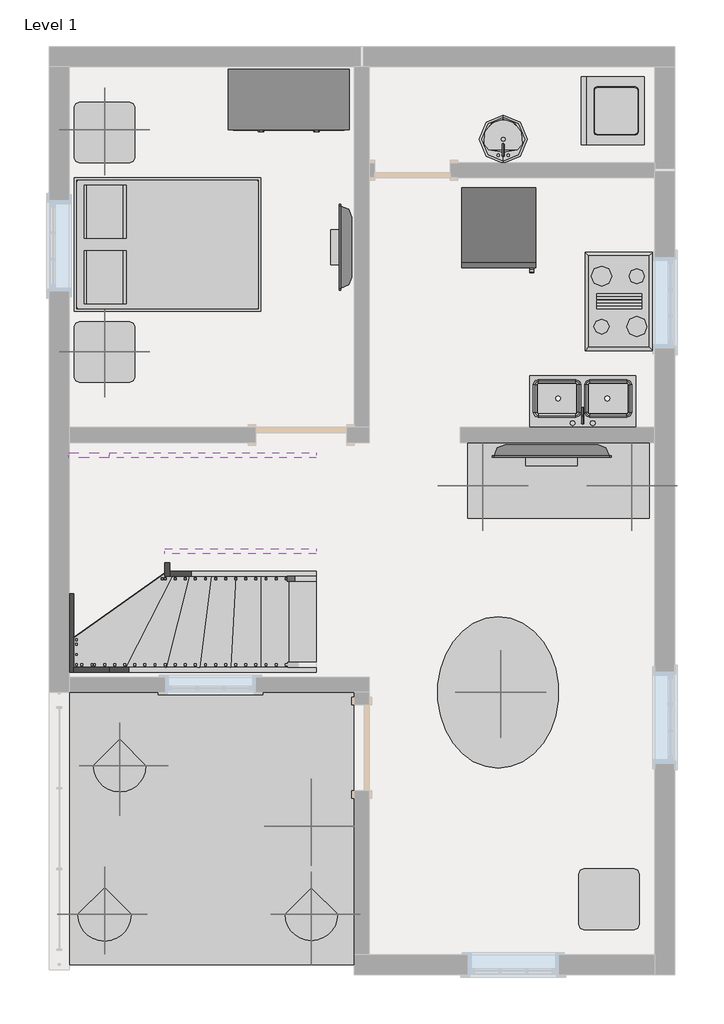
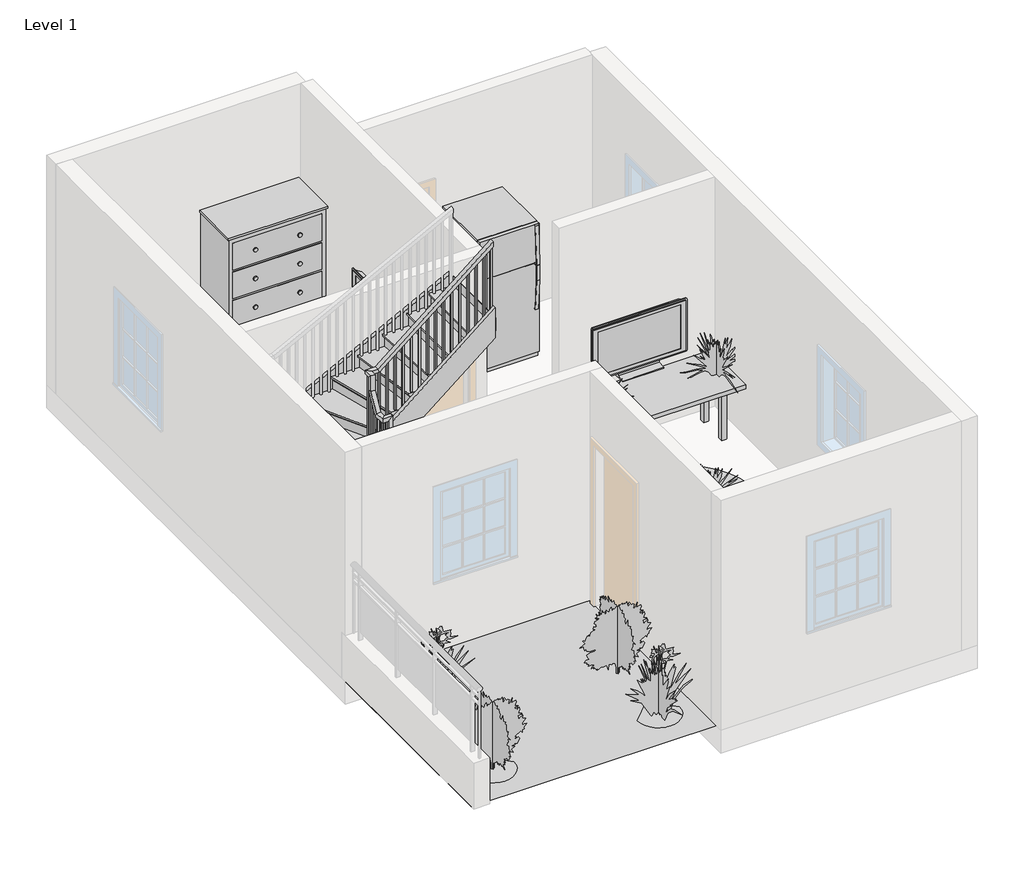
# One storey, part 3 of 3: 9 furniture elements, 9 geographic elements, 8 members, 4 proxies, 3 flow terminals, 1 railing, 1 stair flight.
"""IFC4 building model written with IfcOpenShell, lengths in millimetres."""

from ifc_helpers import new_model, si_unit, frame, origin, place, context, project, spatial, polyline, outline, extrude, faceted_brep, triangles, transform, mapped, element, save
from components import proxy_bb1e6e30, proxy_a13a33b2, proxy_718fa39f, flow_terminal_2b63360b, flow_terminal_a53be723, flow_terminal_d49f872f, furniture_c8abb964, furniture_9fa109b2, furniture_56245f3a, furniture_d9bcc661, furniture_743965d2, furniture_31d08a24, furniture_a5b052b6, rpc_plant_tropical_55f6ff97, rpc_plant_tropical_agave_1_5_93a2a214, rpc_plant_tropical_jungle_flame_3_9c4808c2, stair_flight_e7c1aa98

model = new_model("IFC4")

# Units and contexts
model_context = context("Model", 3, world=origin())
ifc_project = project(units=[si_unit("LENGTHUNIT", "METRE", prefix="MILLI")], contexts=[model_context])

# Site, building, storey
site = spatial("IfcSite", under=ifc_project)
building = spatial("IfcBuilding", under=site)
storey = spatial("IfcBuildingStorey", under=building, Name="Level 1", Elevation=0.0)

# Proxies
placement = place(None, origin())
element("IfcBuildingElementProxy", 1, Name="Building Element Proxy", at=placement, inside=storey, context=model_context, shape_type="Tessellation", body=[
    triangles([(-16784.817334, 6612.6463715, 0.0), (-13559.0165588, 6487.3377411, 0.0), (-13635.2165588, 3869.4466621, 0.0), (-16784.817334, 3869.4466621, 0.0), (-13711.4165588, 6612.6463715, 0.0)], [[1, 4, 5], [5, 3, 2], [3, 5, 4]], closed=False),
])
proxy_shape = proxy_bb1e6e30(model_context)
element("IfcBuildingElementProxy", 2, Name="Cook Top-4 Unit : 36\" x 20\"", ObjectType="Cook Top-4 Unit : 36\" x 20\"", at=placement, inside=storey, context=model_context, shape_type="MappedRepresentation", body=[
    mapped(proxy_shape, transform((-11044.4170266, 10549.6465295, 0.0), x_axis=(0.0, -1.0000000000000004, 0.0), y_axis=(1.0000000000000004, 0.0, 0.0), z_axis=(0.0, 0.0, 1.0))),
])
proxy_2_shape = proxy_a13a33b2(model_context)
element("IfcBuildingElementProxy", 3, Name="Refrigerator : 30\" x 32\" RH", ObjectType="Refrigerator : 30\" x 32\" RH", at=placement, inside=storey, context=model_context, shape_type="MappedRepresentation", body=[
    mapped(proxy_2_shape, transform((-12255.6795266, 11304.097558, 0.0), x_axis=(1.0, 0.0, 0.0), y_axis=(0.0, 1.0, 0.0), z_axis=(0.0, 0.0, 1.0))),
])
proxy_3_shape = proxy_718fa39f(model_context)
element("IfcBuildingElementProxy", 4, Name="Washer : 27\" x 25\" x 35\"", ObjectType="Washer : 27\" x 25\" x 35\"", at=placement, inside=storey, context=model_context, shape_type="MappedRepresentation", body=[
    mapped(proxy_3_shape, transform((-10828.7674618, 12046.929061, 0.0), x_axis=(0.0, 1.0000000000000002, 0.0), y_axis=(-1.0000000000000002, 0.0, 0.0), z_axis=(0.0, 0.0, 1.0))),
])

# Flow terminals
flow_terminal_shape = flow_terminal_2b63360b(model_context)
element("IfcFlowTerminal", 5, ObjectType="Floor Drain - Rectangular : 5\"x5\" Strainer - 2\" Drain", at=placement, inside=storey, context=model_context, shape_type="MappedRepresentation", body=[
    mapped(flow_terminal_shape, transform((-11806.4170266, 12734.0465295, 0.0), x_axis=(1.0, 0.0, 0.0), y_axis=(0.0, 1.0, 0.0), z_axis=(0.0, 0.0, 1.0))),
])
flow_terminal_2_shape = flow_terminal_a53be723(model_context)
element("IfcFlowTerminal", 6, ObjectType="Sink Kitchen-Double : 42\" x 21\"", at=placement, inside=storey, context=model_context, shape_type="MappedRepresentation", body=[
    mapped(flow_terminal_2_shape, transform((-11397.027786, 9535.9919306, 0.0), x_axis=(-1.0, 0.0, 0.0), y_axis=(0.0, -1.0, 0.0), z_axis=(0.0, 0.0, 1.0))),
])
flow_terminal_3_shape = flow_terminal_d49f872f(model_context)
element("IfcFlowTerminal", 7, ObjectType="Sink Vanity-Round : 19\" x 19\"", at=placement, inside=storey, context=model_context, shape_type="MappedRepresentation", body=[
    mapped(flow_terminal_3_shape, transform((-12116.165286, 12267.8503956, 0.0), x_axis=(-1.0000000000000004, 0.0, 0.0), y_axis=(0.0, -1.0000000000000004, 0.0), z_axis=(0.0, 0.0, 1.0))),
])

# Furniture
furniture_shape = furniture_c8abb964(model_context)
element("IfcFurniture", 8, ObjectType="Bed-Box : Double 53\" x 74\"", at=placement, inside=storey, context=model_context, shape_type="MappedRepresentation", body=[
    mapped(furniture_shape, transform((-15825.4465348, 10781.9940704, 0.0), x_axis=(0.0, 1.0, 0.0), y_axis=(-1.0, 0.0, 0.0), z_axis=(0.0, 0.0, 1.0))),
])
furniture_2_shape = furniture_9fa109b2(model_context)
element("IfcFurniture", 9, ObjectType="Dresser : 48\" x 72\" x 24\"", at=placement, inside=storey, context=model_context, shape_type="MappedRepresentation", body=[
    mapped(furniture_2_shape, transform((-14102.6237667, 12944.8094836, 0.0), x_axis=(1.0, 0.0, 0.0), y_axis=(0.0, 1.0, 0.0), z_axis=(0.0, 0.0, 1.0))),
])
furniture_3_shape = furniture_56245f3a(model_context)
element("IfcFurniture", 10, ObjectType="TV - Flat Screen : 32\"", at=placement, inside=storey, context=model_context, shape_type="MappedRepresentation", body=[
    mapped(furniture_3_shape, transform((-13795.3556502, 11091.8020153, 914.4), x_axis=(0.0, -1.0000000000000002, 0.0), y_axis=(1.0000000000000002, 0.0, 0.0), z_axis=(0.0, 0.0, 1.0))),
])
furniture_4_shape = furniture_d9bcc661(model_context)
element("IfcFurniture", 11, ObjectType="TV - Flat Screen : 46\"", at=placement, inside=storey, context=model_context, shape_type="MappedRepresentation", body=[
    mapped(furniture_4_shape, transform((-11719.9225124, 9047.0043586, 914.4), x_axis=(1.0, 0.0, 0.0), y_axis=(0.0, 1.0, 0.0), z_axis=(0.0, 0.0, 1.0))),
])
furniture_5_shape = furniture_743965d2(model_context)
element("IfcFurniture", 12, ObjectType="Table-Ellipse : 60\" x 48\"", at=placement, inside=storey, context=model_context, shape_type="MappedRepresentation", body=[
    mapped(furniture_5_shape, transform((-12263.6170266, 6612.6465295, 0.0), x_axis=(0.0, 1.0000000000000002, 0.0), y_axis=(-1.0000000000000002, 0.0, 0.0), z_axis=(0.0, 0.0, 1.0))),
])
furniture_6_shape = furniture_31d08a24(model_context)
element("IfcFurniture", 13, ObjectType="Table-End : 24\" x 24\"", at=placement, inside=storey, context=model_context, shape_type="MappedRepresentation", body=[
    mapped(furniture_6_shape, transform((-16534.5506569, 9889.2465295, 0.0), x_axis=(1.0, 0.0, 0.0), y_axis=(0.0, 1.0, 0.0), z_axis=(0.0, 0.0, 1.0))),
])
element("IfcFurniture", 14, ObjectType="Table-End : 24\" x 24\"", at=placement, inside=storey, context=model_context, shape_type="MappedRepresentation", body=[
    mapped(furniture_6_shape, transform((-16534.5506569, 12099.0465295, 0.0), x_axis=(1.0, 0.0, 0.0), y_axis=(0.0, 1.0, 0.0), z_axis=(0.0, 0.0, 1.0))),
])
element("IfcFurniture", 15, ObjectType="Table-End : 24\" x 24\"", at=placement, inside=storey, context=model_context, shape_type="MappedRepresentation", body=[
    mapped(furniture_6_shape, transform((-11454.5506569, 4377.4465295, 0.0), x_axis=(1.0, 0.0, 0.0), y_axis=(0.0, 1.0, 0.0), z_axis=(0.0, 0.0, 1.0))),
])
furniture_7_shape = furniture_a5b052b6(model_context)
element("IfcFurniture", 16, ObjectType="Table-Rectangular : 72\" x 30\"", at=placement, inside=storey, context=model_context, shape_type="MappedRepresentation", body=[
    mapped(furniture_7_shape, transform((-11654.0170266, 8746.2465295, 0.0), x_axis=(1.0, 0.0, 0.0), y_axis=(0.0, 1.0, 0.0), z_axis=(0.0, 0.0, 1.0))),
])

# Geographic elements
rpc_plant_tropical_shape = rpc_plant_tropical_55f6ff97(model_context)
element("IfcGeographicElement", 17, ObjectType="RPC Plant - Tropical", at=placement, inside=storey, context=model_context, shape_type="MappedRepresentation", body=[
    mapped(rpc_plant_tropical_shape, transform((-16073.6170266, 5876.0465295, 0.0), x_axis=(1.0, 0.0, 0.0), y_axis=(0.0, 1.0, 0.0), z_axis=(0.0, 0.0, 1.0))),
])
element("IfcGeographicElement", 18, ObjectType="RPC Plant - Tropical", at=placement, inside=storey, context=model_context, shape_type="MappedRepresentation", body=[
    mapped(rpc_plant_tropical_shape, transform((-14143.2170266, 4377.4465295, 0.0), x_axis=(1.0, 0.0, 0.0), y_axis=(0.0, 1.0, 0.0), z_axis=(0.0, 0.0, 1.0))),
])
rpc_plant_tropical_agave_1_5_shape = rpc_plant_tropical_agave_1_5_93a2a214(model_context)
element("IfcGeographicElement", 19, ObjectType="RPC Plant - Tropical : Agave - 1.5'", at=placement, inside=storey, context=model_context, shape_type="MappedRepresentation", body=[
    mapped(rpc_plant_tropical_agave_1_5_shape, transform((-16226.0170266, 12276.8465295, 609.6), x_axis=(1.0, 0.0, 0.0), y_axis=(0.0, 1.0, 0.0), z_axis=(0.0, 0.0, 1.0))),
])
element("IfcGeographicElement", 20, ObjectType="RPC Plant - Tropical : Agave - 1.5'", at=placement, inside=storey, context=model_context, shape_type="MappedRepresentation", body=[
    mapped(rpc_plant_tropical_agave_1_5_shape, transform((-16226.0170266, 10041.6465295, 609.6), x_axis=(1.0, 0.0, 0.0), y_axis=(0.0, 1.0, 0.0), z_axis=(0.0, 0.0, 1.0))),
])
element("IfcGeographicElement", 21, ObjectType="RPC Plant - Tropical : Agave - 1.5'", at=placement, inside=storey, context=model_context, shape_type="MappedRepresentation", body=[
    mapped(rpc_plant_tropical_agave_1_5_shape, transform((-12238.2170266, 6612.6465295, 762.0), x_axis=(1.0, 0.0, 0.0), y_axis=(0.0, 1.0, 0.0), z_axis=(0.0, 0.0, 1.0))),
])
element("IfcGeographicElement", 22, ObjectType="RPC Plant - Tropical : Agave - 1.5'", at=placement, inside=storey, context=model_context, shape_type="MappedRepresentation", body=[
    mapped(rpc_plant_tropical_agave_1_5_shape, transform((-10917.4170266, 8695.4465295, 762.0), x_axis=(1.0, 0.0, 0.0), y_axis=(0.0, 1.0, 0.0), z_axis=(0.0, 0.0, 1.0))),
])
element("IfcGeographicElement", 23, ObjectType="RPC Plant - Tropical : Agave - 1.5'", at=placement, inside=storey, context=model_context, shape_type="MappedRepresentation", body=[
    mapped(rpc_plant_tropical_agave_1_5_shape, transform((-12416.0170266, 8695.4465295, 762.0), x_axis=(1.0, 0.0, 0.0), y_axis=(0.0, 1.0, 0.0), z_axis=(0.0, 0.0, 1.0))),
])
rpc_plant_tropical_jungle_flame_3_shape = rpc_plant_tropical_jungle_flame_3_9c4808c2(model_context)
element("IfcGeographicElement", 24, ObjectType="RPC Plant - Tropical : Jungle Flame - 3'", at=placement, inside=storey, context=model_context, shape_type="MappedRepresentation", body=[
    mapped(rpc_plant_tropical_jungle_flame_3_shape, transform((-16226.0170266, 4377.4465295, 0.0), x_axis=(1.0, 0.0, 0.0), y_axis=(0.0, 1.0, 0.0), z_axis=(0.0, 0.0, 1.0))),
])
element("IfcGeographicElement", 25, ObjectType="RPC Plant - Tropical : Jungle Flame - 3'", at=placement, inside=storey, context=model_context, shape_type="MappedRepresentation", body=[
    mapped(rpc_plant_tropical_jungle_flame_3_shape, transform((-14143.2170266, 5266.4465295, 0.0), x_axis=(1.0, 0.0, 0.0), y_axis=(0.0, 1.0, 0.0), z_axis=(0.0, 0.0, 1.0))),
])

# Members
element("IfcMember", 26, ObjectType="Stringer - 2\" Width", at=placement, inside=storey, context=model_context, shape_type="SweptSolid", body=[
    extrude(outline(polyline([(0.0, -14092.4170266), (229.639954, -14092.4170266), (1305.3956453, -16179.8342183), (962.500629, -16179.8342183), (0.0, -14312.1793441), (0.0, -14092.4170266)])), frame((0.0, 6815.8465295, 0.0), z_axis=(0.0, 1.0, 0.0), x_axis=(0.0, 0.0, 1.0)), (0.0, 0.0, 1.0), 50.8),
])
element("IfcMember", 27, ObjectType="Stringer - 2\" Width", at=placement, inside=storey, context=model_context, shape_type="SweptSolid", body=[
    extrude(outline(polyline([(-16179.8342183, 6866.6465295), (-16179.8342183, 6815.8465295), (-16534.5487184, 6815.8465295), (-16534.5487184, 6866.6465295), (-16179.8342183, 6866.6465295)])), frame((0.0, 0.0, 962.500629), z_axis=(0.0, 0.0, 1.0), x_axis=(1.0, 0.0, 0.0)), (0.0, 0.0, 1.0), 342.8950162),
])
element("IfcMember", 28, ObjectType="Stringer - 2\" Width", at=placement, inside=storey, context=model_context, shape_type="SweptSolid", body=[
    extrude(outline(polyline([(6815.8465295, 1000.5956453), (6815.8465295, 1289.0952212), (8937.8664122, 1969.9972697), (8974.8465295, 1969.9972697), (8974.8465295, 1638.9682298), (6985.3690124, 1000.5956453), (6815.8465295, 1000.5956453)])), frame((-16585.3487184, 0.0, 0.0), z_axis=(1.0, 0.0, 0.0), x_axis=(0.0, 1.0, 0.0)), (0.0, 0.0, 1.0), 50.8),
])
element("IfcMember", 29, ObjectType="Stringer - 2\" Width", at=placement, inside=storey, context=model_context, shape_type="SweptSolid", body=[
    extrude(outline(polyline([(-16585.3487184, 8974.8465295), (-16585.3487184, 9025.6465295), (-16179.8342183, 9025.6465295), (-16179.8342183, 8974.8465295), (-16585.3487184, 8974.8465295)])), frame((0.0, 0.0, 1649.8904473), z_axis=(0.0, 0.0, 1.0), x_axis=(1.0, 0.0, 0.0)), (0.0, 0.0, 1.0), 320.1068224),
])
element("IfcMember", 30, ObjectType="Stringer - 2\" Width", at=placement, inside=storey, context=model_context, shape_type="SweptSolid", body=[
    extrude(outline(polyline([(1969.9972697, -16179.8342183), (1649.8904473, -16179.8342183), (2725.6461385, -14092.4170266), (3045.7529609, -14092.4170266), (1969.9972697, -16179.8342183)])), frame((0.0, 8974.8465295, 0.0), z_axis=(0.0, 1.0, 0.0), x_axis=(0.0, 0.0, 1.0)), (0.0, 0.0, 1.0), 50.8),
])
element("IfcMember", 31, ObjectType="Stringer - 2\" Width", at=placement, inside=storey, context=model_context, shape_type="SweptSolid", body=[
    extrude(outline(polyline([(0.0, -14092.4170266), (176.1764461, -14092.4170266), (1380.418648, -15569.3487184), (987.1410923, -15569.3487184), (0.0, -14358.6786711), (0.0, -14092.4170266)])), frame((0.0, 7781.0465295, 0.0), z_axis=(0.0, 1.0, 0.0), x_axis=(0.0, 0.0, 1.0)), (0.0, 0.0, 1.0), 50.8),
])
element("IfcMember", 32, ObjectType="Stringer - 2\" Width", at=placement, inside=storey, context=model_context, shape_type="SweptSolid", body=[
    extrude(outline(polyline([(7781.0465295, 1028.5617647), (7781.0465295, 1573.2682978), (7987.6836469, 1926.1409689), (8009.6465295, 1926.1409689), (8009.6465295, 1360.465107), (7815.2887468, 1028.5617647), (7781.0465295, 1028.5617647)])), frame((-15620.1487184, 0.0, 0.0), z_axis=(1.0, 0.0, 0.0), x_axis=(0.0, 1.0, 0.0)), (0.0, 0.0, 1.0), 50.8),
])
element("IfcMember", 33, ObjectType="Stringer - 2\" Width", at=placement, inside=storey, context=model_context, shape_type="SweptSolid", body=[
    extrude(outline(polyline([(1926.1409689, -15620.1487184), (1532.8634131, -15620.1487184), (2778.5262875, -14092.4170266), (3171.8038432, -14092.4170266), (1926.1409689, -15620.1487184)])), frame((0.0, 8009.6465295, 0.0), z_axis=(0.0, 1.0, 0.0), x_axis=(0.0, 0.0, 1.0)), (0.0, 0.0, 1.0), 50.8),
])

# Railing
element("IfcRailing", 34, ObjectType="Handrail - Rectangular", at=placement, inside=storey, context=model_context, shape_type="SolidModel", body=[
    faceted_brep([(-14092.4170266, 7730.2465295, 1025.2529681), (-14092.4170266, 7730.2465295, 959.7067088), (-14092.4170266, 7781.0465295, 959.7067088), (-14092.4170266, 7781.0465295, 1025.2529681), (-15543.9487184, 7730.2465295, 2208.7848338), (-15594.7487184, 7730.2465295, 2184.659247), (-15594.7487184, 7781.0465295, 2184.659247), (-15543.9487184, 7781.0465295, 2208.7848338), (-15543.9487184, 7730.2465295, 2414.6281882), (-15594.7487184, 7730.2465295, 2363.8281882), (-15594.7487184, 7781.0465295, 2363.8281882), (-15543.9487184, 7781.0465295, 2414.6281882), (-15670.9487184, 7730.2465295, 2414.6281882), (-15670.9487184, 7730.2465295, 2363.8281882), (-15620.1487184, 7781.0465295, 2363.8281882), (-15620.1487184, 7781.0465295, 2414.6281882), (-15670.9487184, 7857.2465295, 2414.6281882), (-15670.9487184, 7886.3678633, 2363.8281882), (-15620.1487184, 7886.3678633, 2363.8281882), (-15620.1487184, 7857.2465295, 2414.6281882), (-15670.9487184, 7984.2465295, 2631.5051451), (-15670.9487184, 8035.0465295, 2617.7256424), (-15620.1487184, 8035.0465295, 2617.7256424), (-15620.1487184, 7984.2465295, 2631.5051451), (-15670.9487184, 7984.2465295, 2837.3484995), (-15670.9487184, 8035.0465295, 2786.5484995), (-15620.1487184, 8035.0465295, 2786.5484995), (-15620.1487184, 7984.2465295, 2837.3484995), (-15670.9487184, 8111.2465295, 2837.3484995), (-15670.9487184, 8111.2465295, 2786.5484995), (-15620.1487184, 8060.4465295, 2786.5484995), (-15620.1487184, 8060.4465295, 2837.3484995), (-15543.9487184, 8111.2465295, 2837.3484995), (-15525.8633053, 8111.2465295, 2786.5484995), (-15525.8633053, 8060.4465295, 2786.5484995), (-15543.9487184, 8060.4465295, 2837.3484995), (-14092.4170266, 8111.2465295, 4020.8803652), (-14092.4170266, 8060.4465295, 4020.8803652), (-14092.4170266, 8060.4465295, 3955.3341059), (-14092.4170266, 8111.2465295, 3955.3341059)], [[[0, 1, 2, 3]], [[1, 0, 4, 5]], [[2, 1, 5, 6]], [[3, 2, 6, 7]], [[0, 3, 7, 4]], [[5, 4, 8, 9]], [[6, 5, 9, 10]], [[7, 6, 10, 11]], [[4, 7, 11, 8]], [[9, 8, 12, 13]], [[10, 9, 13, 14]], [[11, 10, 14, 15]], [[8, 11, 15, 12]], [[13, 12, 16, 17]], [[14, 13, 17, 18]], [[15, 14, 18, 19]], [[12, 15, 19, 16]], [[17, 16, 20, 21]], [[18, 17, 21, 22]], [[19, 18, 22, 23]], [[16, 19, 23, 20]], [[21, 20, 24, 25]], [[22, 21, 25, 26]], [[23, 22, 26, 27]], [[20, 23, 27, 24]], [[25, 24, 28, 29]], [[26, 25, 29, 30]], [[27, 26, 30, 31]], [[24, 27, 31, 28]], [[29, 28, 32, 33]], [[30, 29, 33, 34]], [[31, 30, 34, 35]], [[28, 31, 35, 32]], [[36, 37, 38, 39]], [[33, 32, 36, 39]], [[34, 33, 39, 38]], [[35, 34, 38, 37]], [[32, 35, 37, 36]]]),
    extrude(outline(polyline([(3881.7558784, -14182.6563621), (3866.2231262, -14201.7063621), (2878.6666667, -14201.7063621), (2878.6666667, -14182.6563621), (3881.7558784, -14182.6563621)])), frame((0.0, 8076.3215295, 0.0), z_axis=(0.0, 1.0, 0.0), x_axis=(0.0, 0.0, 1.0)), (0.0, 0.0, 1.0), 19.05),
    extrude(outline(polyline([(3798.9145334, -14284.2563621), (3783.3817813, -14303.3063621), (2878.6666667, -14303.3063621), (2878.6666667, -14284.2563621), (3798.9145334, -14284.2563621)])), frame((0.0, 8076.3215295, 0.0), z_axis=(0.0, 1.0, 0.0), x_axis=(0.0, 0.0, 1.0)), (0.0, 0.0, 1.0), 19.05),
    extrude(outline(polyline([(3716.0731885, -14385.8563621), (3700.5404364, -14404.9063621), (2709.3333333, -14404.9063621), (2709.3333333, -14385.8563621), (3716.0731885, -14385.8563621)])), frame((0.0, 8076.3215295, 0.0), z_axis=(0.0, 1.0, 0.0), x_axis=(0.0, 0.0, 1.0)), (0.0, 0.0, 1.0), 19.05),
    extrude(outline(polyline([(3633.2318436, -14487.4563621), (3617.6990914, -14506.5063621), (2709.3333333, -14506.5063621), (2709.3333333, -14487.4563621), (3633.2318436, -14487.4563621)])), frame((0.0, 8076.3215295, 0.0), z_axis=(0.0, 1.0, 0.0), x_axis=(0.0, 0.0, 1.0)), (0.0, 0.0, 1.0), 19.05),
    extrude(outline(polyline([(3550.3904987, -14589.0563621), (3534.8577465, -14608.1063621), (2709.3333333, -14608.1063621), (2709.3333333, -14589.0563621), (3550.3904987, -14589.0563621)])), frame((0.0, 8076.3215295, 0.0), z_axis=(0.0, 1.0, 0.0), x_axis=(0.0, 0.0, 1.0)), (0.0, 0.0, 1.0), 19.05),
    extrude(outline(polyline([(3467.5491538, -14690.6563621), (3452.0164016, -14709.7063621), (2540.0, -14709.7063621), (2540.0, -14690.6563621), (3467.5491538, -14690.6563621)])), frame((0.0, 8076.3215295, 0.0), z_axis=(0.0, 1.0, 0.0), x_axis=(0.0, 0.0, 1.0)), (0.0, 0.0, 1.0), 19.05),
    extrude(outline(polyline([(3384.7078088, -14792.2563621), (3369.1750567, -14811.3063621), (2540.0, -14811.3063621), (2540.0, -14792.2563621), (3384.7078088, -14792.2563621)])), frame((0.0, 8076.3215295, 0.0), z_axis=(0.0, 1.0, 0.0), x_axis=(0.0, 0.0, 1.0)), (0.0, 0.0, 1.0), 19.05),
    extrude(outline(polyline([(3301.8664639, -14893.8563621), (3286.3337117, -14912.9063621), (2540.0, -14912.9063621), (2540.0, -14893.8563621), (3301.8664639, -14893.8563621)])), frame((0.0, 8076.3215295, 0.0), z_axis=(0.0, 1.0, 0.0), x_axis=(0.0, 0.0, 1.0)), (0.0, 0.0, 1.0), 19.05),
    extrude(outline(polyline([(3219.025119, -14995.4563621), (3203.4923668, -15014.5063621), (2370.6666667, -15014.5063621), (2370.6666667, -14995.4563621), (3219.025119, -14995.4563621)])), frame((0.0, 8076.3215295, 0.0), z_axis=(0.0, 1.0, 0.0), x_axis=(0.0, 0.0, 1.0)), (0.0, 0.0, 1.0), 19.05),
    extrude(outline(polyline([(3136.1837741, -15097.0563621), (3120.6510219, -15116.1063621), (2370.6666667, -15116.1063621), (2370.6666667, -15097.0563621), (3136.1837741, -15097.0563621)])), frame((0.0, 8076.3215295, 0.0), z_axis=(0.0, 1.0, 0.0), x_axis=(0.0, 0.0, 1.0)), (0.0, 0.0, 1.0), 19.05),
    extrude(outline(polyline([(3053.3424291, -15198.6563621), (3037.809677, -15217.7063621), (2201.3333333, -15217.7063621), (2201.3333333, -15198.6563621), (3053.3424291, -15198.6563621)])), frame((0.0, 8076.3215295, 0.0), z_axis=(0.0, 1.0, 0.0), x_axis=(0.0, 0.0, 1.0)), (0.0, 0.0, 1.0), 19.05),
    extrude(outline(polyline([(2970.5010842, -15300.2563621), (2954.9683321, -15319.3063621), (2201.3333333, -15319.3063621), (2201.3333333, -15300.2563621), (2970.5010842, -15300.2563621)])), frame((0.0, 8076.3215295, 0.0), z_axis=(0.0, 1.0, 0.0), x_axis=(0.0, 0.0, 1.0)), (0.0, 0.0, 1.0), 19.05),
    extrude(outline(polyline([(2887.6597393, -15401.8563621), (2872.1269871, -15420.9063621), (2032.0, -15420.9063621), (2032.0, -15401.8563621), (2887.6597393, -15401.8563621)])), frame((0.0, 8076.3215295, 0.0), z_axis=(0.0, 1.0, 0.0), x_axis=(0.0, 0.0, 1.0)), (0.0, 0.0, 1.0), 19.05),
    extrude(outline(polyline([(2804.8183944, -15503.4563621), (2789.2856422, -15522.5063621), (2032.0, -15522.5063621), (2032.0, -15503.4563621), (2804.8183944, -15503.4563621)])), frame((0.0, 8076.3215295, 0.0), z_axis=(0.0, 1.0, 0.0), x_axis=(0.0, 0.0, 1.0)), (0.0, 0.0, 1.0), 19.05),
    extrude(outline(polyline([(7964.1074332, 2496.5834745), (7983.1574332, 2529.115018), (7983.1574332, 1524.0), (7964.1074332, 1524.0), (7964.1074332, 2496.5834745)])), frame((-15655.0737184, 0.0, 0.0), z_axis=(1.0, 0.0, 0.0), x_axis=(0.0, 1.0, 0.0)), (0.0, 0.0, 1.0), 19.05),
    extrude(outline(polyline([(7862.5074332, 2323.0819089), (7881.5574332, 2355.6134525), (7881.5574332, 1524.0), (7862.5074332, 1524.0), (7862.5074332, 2323.0819089)])), frame((-15655.0737184, 0.0, 0.0), z_axis=(1.0, 0.0, 0.0), x_axis=(0.0, 1.0, 0.0)), (0.0, 0.0, 1.0), 19.05),
    extrude(outline(polyline([(2111.7191617, -15505.2920266), (2127.2519138, -15524.3420266), (1016.0, -15524.3420266), (1016.0, -15505.2920266), (2111.7191617, -15505.2920266)])), frame((0.0, 7746.1215295, 0.0), z_axis=(0.0, 1.0, 0.0), x_axis=(0.0, 0.0, 1.0)), (0.0, 0.0, 1.0), 19.05),
    extrude(outline(polyline([(2028.8778167, -15403.6920266), (2044.4105689, -15422.7420266), (1016.0, -15422.7420266), (1016.0, -15403.6920266), (2028.8778167, -15403.6920266)])), frame((0.0, 7746.1215295, 0.0), z_axis=(0.0, 1.0, 0.0), x_axis=(0.0, 0.0, 1.0)), (0.0, 0.0, 1.0), 19.05),
    extrude(outline(polyline([(1946.0364718, -15302.0920266), (1961.569224, -15321.1420266), (846.6666667, -15321.1420266), (846.6666667, -15302.0920266), (1946.0364718, -15302.0920266)])), frame((0.0, 7746.1215295, 0.0), z_axis=(0.0, 1.0, 0.0), x_axis=(0.0, 0.0, 1.0)), (0.0, 0.0, 1.0), 19.05),
    extrude(outline(polyline([(1863.1951269, -15200.4920266), (1878.7278791, -15219.5420266), (846.6666667, -15219.5420266), (846.6666667, -15200.4920266), (1863.1951269, -15200.4920266)])), frame((0.0, 7746.1215295, 0.0), z_axis=(0.0, 1.0, 0.0), x_axis=(0.0, 0.0, 1.0)), (0.0, 0.0, 1.0), 19.05),
    extrude(outline(polyline([(1780.353782, -15098.8920266), (1795.8865341, -15117.9420266), (677.3333333, -15117.9420266), (677.3333333, -15098.8920266), (1780.353782, -15098.8920266)])), frame((0.0, 7746.1215295, 0.0), z_axis=(0.0, 1.0, 0.0), x_axis=(0.0, 0.0, 1.0)), (0.0, 0.0, 1.0), 19.05),
    extrude(outline(polyline([(1697.5124371, -14997.2920266), (1713.0451892, -15016.3420266), (677.3333333, -15016.3420266), (677.3333333, -14997.2920266), (1697.5124371, -14997.2920266)])), frame((0.0, 7746.1215295, 0.0), z_axis=(0.0, 1.0, 0.0), x_axis=(0.0, 0.0, 1.0)), (0.0, 0.0, 1.0), 19.05),
    extrude(outline(polyline([(1614.6710921, -14895.6920266), (1630.2038443, -14914.7420266), (508.0, -14914.7420266), (508.0, -14895.6920266), (1614.6710921, -14895.6920266)])), frame((0.0, 7746.1215295, 0.0), z_axis=(0.0, 1.0, 0.0), x_axis=(0.0, 0.0, 1.0)), (0.0, 0.0, 1.0), 19.05),
    extrude(outline(polyline([(1531.8297472, -14794.0920266), (1547.3624994, -14813.1420266), (508.0, -14813.1420266), (508.0, -14794.0920266), (1531.8297472, -14794.0920266)])), frame((0.0, 7746.1215295, 0.0), z_axis=(0.0, 1.0, 0.0), x_axis=(0.0, 0.0, 1.0)), (0.0, 0.0, 1.0), 19.05),
    extrude(outline(polyline([(1448.9884023, -14692.4920266), (1464.5211545, -14711.5420266), (508.0, -14711.5420266), (508.0, -14692.4920266), (1448.9884023, -14692.4920266)])), frame((0.0, 7746.1215295, 0.0), z_axis=(0.0, 1.0, 0.0), x_axis=(0.0, 0.0, 1.0)), (0.0, 0.0, 1.0), 19.05),
    extrude(outline(polyline([(1366.1470574, -14590.8920266), (1381.6798095, -14609.9420266), (338.6666667, -14609.9420266), (338.6666667, -14590.8920266), (1366.1470574, -14590.8920266)])), frame((0.0, 7746.1215295, 0.0), z_axis=(0.0, 1.0, 0.0), x_axis=(0.0, 0.0, 1.0)), (0.0, 0.0, 1.0), 19.05),
    extrude(outline(polyline([(1283.3057124, -14489.2920266), (1298.8384646, -14508.3420266), (338.6666667, -14508.3420266), (338.6666667, -14489.2920266), (1283.3057124, -14489.2920266)])), frame((0.0, 7746.1215295, 0.0), z_axis=(0.0, 1.0, 0.0), x_axis=(0.0, 0.0, 1.0)), (0.0, 0.0, 1.0), 19.05),
    extrude(outline(polyline([(1200.4643675, -14387.6920266), (1215.9971197, -14406.7420266), (338.6666667, -14406.7420266), (338.6666667, -14387.6920266), (1200.4643675, -14387.6920266)])), frame((0.0, 7746.1215295, 0.0), z_axis=(0.0, 1.0, 0.0), x_axis=(0.0, 0.0, 1.0)), (0.0, 0.0, 1.0), 19.05),
    extrude(outline(polyline([(1117.6230226, -14286.0920266), (1133.1557748, -14305.1420266), (169.3333333, -14305.1420266), (169.3333333, -14286.0920266), (1117.6230226, -14286.0920266)])), frame((0.0, 7746.1215295, 0.0), z_axis=(0.0, 1.0, 0.0), x_axis=(0.0, 0.0, 1.0)), (0.0, 0.0, 1.0), 19.05),
    extrude(outline(polyline([(1034.7816777, -14184.4920266), (1050.3144298, -14203.5420266), (169.3333333, -14203.5420266), (169.3333333, -14184.4920266), (1034.7816777, -14184.4920266)])), frame((0.0, 7746.1215295, 0.0), z_axis=(0.0, 1.0, 0.0), x_axis=(0.0, 0.0, 1.0)), (0.0, 0.0, 1.0), 19.05),
    extrude(outline(polyline([(-15624.1063621, 8076.3215295), (-15624.1063621, 8095.3715295), (-15605.0563621, 8095.3715295), (-15605.0563621, 8076.3215295), (-15624.1063621, 8076.3215295)])), frame((0.0, 0.0, 1862.6666667), z_axis=(0.0, 0.0, 1.0), x_axis=(1.0, 0.0, 0.0)), (0.0, 0.0, 1.0), 923.8818329),
    extrude(outline(polyline([(-15636.0237184, 8076.3215295), (-15655.0737184, 8076.3215295), (-15655.0737184, 8095.3715295), (-15636.0237184, 8095.3715295), (-15636.0237184, 8076.3215295)])), frame((0.0, 0.0, 1862.6666667), z_axis=(0.0, 0.0, 1.0), x_axis=(1.0, 0.0, 0.0)), (0.0, 0.0, 1.0), 923.8818329),
    extrude(outline(polyline([(-15636.0237184, 8061.5356257), (-15655.0737184, 8061.5356257), (-15655.0737184, 8080.5856257), (-15636.0237184, 8080.5856257), (-15636.0237184, 8061.5356257)])), frame((0.0, 0.0, 1693.3333333), z_axis=(0.0, 0.0, 1.0), x_axis=(1.0, 0.0, 0.0)), (0.0, 0.0, 1.0), 1093.2151662),
    extrude(outline(polyline([(-15636.0237184, 7760.9074332), (-15655.0737184, 7760.9074332), (-15655.0737184, 7779.9574332), (-15636.0237184, 7779.9574332), (-15636.0237184, 7760.9074332)])), frame((0.0, 0.0, 1354.6666667), z_axis=(0.0, 0.0, 1.0), x_axis=(1.0, 0.0, 0.0)), (0.0, 0.0, 1.0), 1009.1615215),
    extrude(outline(polyline([(-15636.0237184, 7765.1715295), (-15636.0237184, 7746.1215295), (-15655.0737184, 7746.1215295), (-15655.0737184, 7765.1715295), (-15636.0237184, 7765.1715295)])), frame((0.0, 0.0, 1185.3333333), z_axis=(0.0, 0.0, 1.0), x_axis=(1.0, 0.0, 0.0)), (0.0, 0.0, 1.0), 1178.4948549),
    extrude(outline(polyline([(-15605.0563621, 7765.1715295), (-15605.0563621, 7746.1215295), (-15624.1063621, 7746.1215295), (-15624.1063621, 7765.1715295), (-15605.0563621, 7765.1715295)])), frame((0.0, 0.0, 1185.3333333), z_axis=(0.0, 0.0, 1.0), x_axis=(1.0, 0.0, 0.0)), (0.0, 0.0, 1.0), 1178.4948549),
    extrude(outline(polyline([(3955.3341059, -14092.4170266), (3939.8013537, -14111.4670266), (2878.6666667, -14111.4670266), (2878.6666667, -14092.4170266), (3955.3341059, -14092.4170266)])), frame((0.0, 8076.3215295, 0.0), z_axis=(0.0, 1.0, 0.0), x_axis=(0.0, 0.0, 1.0)), (0.0, 0.0, 1.0), 19.05),
    extrude(outline(polyline([(959.7067088, -14092.4170266), (975.239461, -14111.4670266), (169.3333333, -14111.4670266), (169.3333333, -14092.4170266), (959.7067088, -14092.4170266)])), frame((0.0, 7746.1215295, 0.0), z_axis=(0.0, 1.0, 0.0), x_axis=(0.0, 0.0, 1.0)), (0.0, 0.0, 1.0), 19.05),
])

# Stair flight
stair_flight_shape = stair_flight_e7c1aa98(model_context)
element("IfcStairFlight", 35, ObjectType="2\" Tread 1\" Nosing 1/4\" Riser", at=placement, inside=storey, context=model_context, shape_type="MappedRepresentation", body=[
    mapped(stair_flight_shape, transform((0.0, 0.0, 0.0), x_axis=(1.0, 0.0, 0.0), y_axis=(0.0, 1.0, 0.0), z_axis=(0.0, 0.0, 1.0))),
])

save(model, "model.ifc")

# Revit data of these elements
# Type "Cook Top-4 Unit : 36\" x 20\""
#   Assembly Code = "E1090400"
#   Depth = 2' - 0"
#   Width = 3' - 0"
#   Burner Material = Steel, Chrome Plated
#   Cooktop Material = Steel, Polished
#   Default Elevation = 0
# Type "Refrigerator : 30\" x 32\" RH"
#   Label = "REF."
#   Assembly Code = "E1090400"
#   Depth = 2' - 7 3/4"
#   Handle = 2' - 3"
#   Height = 5' - 10"
#   Rear Clearance = 0' - 2"
#   Top Door Height = 1' - 8"
#   Width = 2' - 5 3/8"
#   Material = Steel, Paint Finish, Ivory, Glossy
#   Default Elevation = 0
# Type "Washer : 27\" x 25\" x 35\""
#   Label = "W"
#   Assembly Code = "E1090400"
#   Depth = 2' - 1"
#   Height = 2' - 11"
#   Width = 2' - 3"
#   Washer Material = Steel, Paint Finish, Ivory, Matte
#   Default Elevation = 0
# Type "Floor Drain - Rectangular : 5\"x5\" Strainer - 2\" Drain"
#   WFU = 2
#   Strainer Height = 0' - 3 1/4"
#   Half Strainer Length = 0' - 2 1/2"
#   Strainer Length = 0' - 5"
#   Radius 2 = 0' - 3.04167"
#   Radius 1 = 0' - 2.02083"
#   Radius 3 = 0' - 2 1/32"
#   Pipe Radius = 1"
#   Pipe Diameter = 2"
#   Height 2 = 0' - 0.725"
#   Height 1 = 0' - 1 13/16"
#   Body Radius = 0' - 4 1/16"
#   Body Height = 0' - 3 5/8"
#   Body Diameter = 0' - 8 1/8"
#   Drain Material = none
#   HWFU = 0
#   Default Elevation = 0
#   CWFU = 0
# Type "Sink Kitchen-Double : 42\" x 21\""
#   Assembly Code = "D2010410"
#   Counter Height = 3' - 0"
#   Depth = 1' - 9"
#   Width = 3' - 6"
#   Faucet Material = Steel, Polished
#   Sink Material = Steel, Polished
#   Default Elevation = 0
# Type "Sink Vanity-Round : 19\" x 19\""
#   Assembly Code = "D2010400"
#   Top Of Counter = 2' - 7"
#   Basin Material = Porcelain, Linen
#   Faucet Material = Steel, Polished
#   Default Elevation = 0
# Type "Bed-Box : Double 53\" x 74\""
#   Assembly Code = "E2020200"
#   Length = 6' - 2"
#   Width = 4' - 5"
#   Frame Material = Birch
#   Mattress Material = Linen, White
#   Default Elevation = 0
# Type "Dresser : 48\" x 72\" x 24\""
#   Assembly Code = "E2020200"
#   Depth = 2' - 0"
#   Height = 6' - 0"
#   Width = 4' - 0"
#   Dresser Material = Laminate - Ivory, Glossy
#   Drawer Material = Laminate, Ivory, Matte
#   Knob Material = Cherry
#   Default Elevation = 0
# Type "TV - Flat Screen : 32\""
#   SinAng = 0' - 0.0193"
#   L = 2' - 3.79372"
#   H = 1' - 3.6354"
#   Thickness = 0' - 4.33071"
#   Diagonal = 2' - 7.88976"
#   CosAng = 0' - 0.03431"
#   Stand [instance default] = yes
#   Default Elevation = 0
# Type "TV - Flat Screen : 46\""
#   SinAng = 0' - 0.0193"
#   L = 3' - 4.83276"
#   H = 1' - 10.97053"
#   Thickness = 0' - 4.33071"
#   Diagonal = 3' - 10.85039"
#   CosAng = 0' - 0.03431"
#   Stand [instance default] = yes
#   Default Elevation = 0
# Type "Table-Ellipse : 60\" x 48\""
#   Assembly Code = "E2020200"
#   Half Width = 2' - 0"
#   Half Length = 2' - 6"
#   Height = 2' - 6"
#   Length = 5' - 0"
#   Width = 4' - 0"
#   Base Material = Birch
#   Top Material = Birch
#   Default Elevation = 0
# Type "Table-End : 24\" x 24\""
#   Assembly Code = "E2020200"
#   Height = 2' - 0"
#   Length = 2' - 0"
#   Width = 2' - 0"
#   Base Material = Birch
#   Top Material = Laminate, Ivory, Matte
#   Default Elevation = 0
# Type "Table-Rectangular : 72\" x 30\""
#   Assembly Code = "E2020200"
#   Height = 2' - 6"
#   Length = 6' - 0"
#   Width = 2' - 6"
#   Base Material = Birch
#   Top Material = Birch
#   Default Elevation = 0
# Type "RPC Plant - Tropical"
#   built-in parameter 1005198 = "{2, 15},{39, RPC-16-FWM5-GM7X-C67P-4000-ST1L-LVER-AU},{1, 0},{1, 0},{2, 13},{1, 8},{5, Color},{1, 0},{1, 0},{3, 0.8},{3, 0.8},{3, 0.8},{1, 8},{7, BBoxMin},{1, 0},{1, 0},{1, 0},{1, 0},{1, 0},{1, 8},{7, BBoxMax},{1, 0},{1, 0},{1, 0},{1, 0},{1, 0},{2, 11},{9, RPCTypeId},{1, 0},{1, 0},{39, RPC-16-FWM5-GM7X-C67P-4000-ST1L-LVER-AU},{1, 6},{14, RPCPlantHeight},{1, 0},{1, 0},{1, 3},{2, 11},{7, keyword},{1, 0},{1, 0},{35, :RPCs:Shrubs [General]:Geometry:RPC},{2, 11},{8, category},{1, 0},{1, 0},{16, Shrubs [General]},{2, 11},{12, LocalizedUID},{1, 0},{1, 0},{10, Crane Lily},{2, 14},{6, Height},{1, 0},{1, 0},{1, 3},{1, 2},{16, Cast Reflections},{1, 0},{1, 0},{1, 0},{1, 2},{12, Cast Shadows},{1, 0},{1, 0},{1, 1},{1, 2},{9, Lock View},{1, 0},{1, 0},{1, 0},{1, 4},{5, ViewC},{1, 0},{1, 0},{1, 0},{21, assetlibrary_base.fbx},{1, 5},"
#   built-in parameter 1005195 = "RPC-16-FWM5-GM7X-C67P-4000-ST1L-LVER-AU"
#   Assembly Code = "G2050500"
#   Height = 3' - 0"
#   Default Elevation = 0
# Type "RPC Plant - Tropical : Agave - 1.5'"
#   built-in parameter 1005198 = "{2, 15},{39, RPC-16-G1GJ-63FX-7K5P-N000-ST1L-LVER-AU},{1, 0},{1, 0},{2, 13},{1, 8},{5, Color},{1, 0},{1, 0},{3, 0.8},{3, 0.8},{3, 0.8},{1, 8},{7, BBoxMin},{1, 0},{1, 0},{1, 0},{1, 0},{1, 0},{1, 8},{7, BBoxMax},{1, 0},{1, 0},{1, 0},{1, 0},{1, 0},{2, 11},{9, RPCTypeId},{1, 0},{1, 0},{39, RPC-16-G1GJ-63FX-7K5P-N000-ST1L-LVER-AU},{1, 6},{14, RPCPlantHeight},{1, 0},{1, 0},{3, 1.5},{2, 11},{7, keyword},{1, 0},{1, 0},{35, :RPCs:Plants [General]:Geometry:RPC},{2, 11},{8, category},{1, 0},{1, 0},{16, Plants [General]},{2, 11},{12, LocalizedUID},{1, 0},{1, 0},{5, Agave},{2, 14},{6, Height},{1, 0},{1, 0},{3, 1.5},{1, 2},{16, Cast Reflections},{1, 0},{1, 0},{1, 0},{1, 2},{12, Cast Shadows},{1, 0},{1, 0},{1, 1},{1, 2},{9, Lock View},{1, 0},{1, 0},{1, 0},{1, 4},{5, ViewC},{1, 0},{1, 0},{1, 0},{21, assetlibrary_base.fbx},{1, 5},"
#   built-in parameter 1005195 = "RPC-16-G1GJ-63FX-7K5P-N000-ST1L-LVER-AU"
#   Type Comments = "Agave"
#   Assembly Code = "G2050500"
#   Height = 1' - 6"
#   Default Elevation = 0
# Type "RPC Plant - Tropical : Jungle Flame - 3'"
#   built-in parameter 1005198 = "{2, 15},{39, RPC-16-FUVJ-JWG0-MWGK-8000-ST1L-LVER-AU},{1, 0},{1, 0},{2, 13},{1, 8},{5, Color},{1, 0},{1, 0},{3, 0.8},{3, 0.8},{3, 0.8},{1, 8},{7, BBoxMin},{1, 0},{1, 0},{1, 0},{1, 0},{1, 0},{1, 8},{7, BBoxMax},{1, 0},{1, 0},{1, 0},{1, 0},{1, 0},{2, 11},{9, RPCTypeId},{1, 0},{1, 0},{39, RPC-16-FUVJ-JWG0-MWGK-8000-ST1L-LVER-AU},{1, 6},{14, RPCPlantHeight},{1, 0},{1, 0},{1, 3},{2, 11},{7, keyword},{1, 0},{1, 0},{35, :RPCs:Shrubs [General]:Geometry:RPC},{2, 11},{8, category},{1, 0},{1, 0},{16, Shrubs [General]},{2, 11},{12, LocalizedUID},{1, 0},{1, 0},{12, Jungle Flame},{2, 14},{6, Height},{1, 0},{1, 0},{1, 3},{1, 2},{16, Cast Reflections},{1, 0},{1, 0},{1, 0},{1, 2},{12, Cast Shadows},{1, 0},{1, 0},{1, 1},{1, 2},{9, Lock View},{1, 0},{1, 0},{1, 0},{1, 4},{5, ViewC},{1, 0},{1, 0},{1, 0},{21, assetlibrary_base.fbx},{1, 5},"
#   built-in parameter 1005195 = "RPC-16-FUVJ-JWG0-MWGK-8000-ST1L-LVER-AU"
#   Type Comments = "Jungle Flame"
#   Assembly Code = "G2050500"
#   Height = 3' - 0"
#   Default Elevation = 0
# Type "Handrail - Rectangular"
#   Assembly Code = "C2010400"
#   built-in parameter 1008612 = 0.0416667 (stored number, unit not read)
#   built-in parameter 1008611 = 0.0416667 (stored number, unit not read)
#   built-in parameter 1008609 = 0.333333 (stored number, unit not read)
#   built-in parameter 1008604 = 0.166667 (stored number, unit not read)
#   built-in parameter 1008603 = 0.166667 (stored number, unit not read)
#   Railing Height = 3' - 0"
#   built-in parameter 1008630 = 2
#   built-in parameter 1008610 = 2
#   built-in parameter 1008618 = Baluster - Square : 3/4"
# Element 1 (IfcBuildingElementProxy)
#   Material = none
#   Phase Created = New Construction
# Element 2 (IfcBuildingElementProxy, "Cook Top-4 Unit : 36\" x 20\"")
#   Phase Created = New Construction
#   Materials on its faces: "Steel, Chrome Plated", "Steel, Polished"
# Element 3 (IfcBuildingElementProxy, "Refrigerator : 30\" x 32\" RH")
#   Phase Created = New Construction
#   Materials on its faces: "Steel, Paint Finish, Ivory, Glossy", "Steel, Chrome Plated"
# Element 4 (IfcBuildingElementProxy, "Washer : 27\" x 25\" x 35\"")
#   Phase Created = New Construction
#   Materials on its faces: "Steel, Paint Finish, Ivory, Matte"
# Element 5 (IfcFlowTerminal, "Floor Drain - Rectangular : 5\"x5\" Strainer - 2\" Drain")
#   Mark = "2"
#   Phase Created = New Construction
# Element 6 (IfcFlowTerminal, "Sink Kitchen-Double : 42\" x 21\"")
#   Mark = "3"
#   Phase Created = New Construction
#   Materials on its faces: "Steel, Polished"
# Element 7 (IfcFlowTerminal, "Sink Vanity-Round : 19\" x 19\"")
#   Mark = "1"
#   Phase Created = New Construction
#   Materials on its faces: "Porcelain, Linen", "Steel, Polished"
# Element 8 (IfcFurniture, "Bed-Box : Double 53\" x 74\"")
#   Phase Created = New Construction
#   Materials on its faces: "Birch", "Linen, White"
# Element 9 (IfcFurniture, "Dresser : 48\" x 72\" x 24\"")
#   Phase Created = New Construction
#   Materials on its faces: "Laminate, Ivory, Matte", "Cherry", "Laminate - Ivory, Glossy"
# Element 10 (IfcFurniture, "TV - Flat Screen : 32\"")
#   Stand = yes
#   Phase Created = New Construction
#   Materials on its faces: "TV - Black", "TV - Glass", "TV - Screen"
# Element 11 (IfcFurniture, "TV - Flat Screen : 46\"")
#   Stand = yes
#   Phase Created = New Construction
#   Materials on its faces: "TV - Black", "TV - Glass", "TV - Screen"
# Element 12 (IfcFurniture, "Table-Ellipse : 60\" x 48\"")
#   Phase Created = New Construction
#   Materials on its faces: "Birch"
# Elements 13, 14, 15 (IfcFurniture, "Table-End : 24\" x 24\"")
#   Phase Created = New Construction
#   Materials on its faces: "Laminate, Ivory, Matte", "Birch"
# Element 16 (IfcFurniture, "Table-Rectangular : 72\" x 30\"")
#   Phase Created = New Construction
#   Materials on its faces: "Birch"
# Elements 17, 18 (IfcGeographicElement, "RPC Plant - Tropical")
#   Phase Created = New Construction
# Elements 19, 20, 21, 22, 23 (IfcGeographicElement, "RPC Plant - Tropical : Agave - 1.5'")
#   Phase Created = New Construction
# Elements 24, 25 (IfcGeographicElement, "RPC Plant - Tropical : Jungle Flame - 3'")
#   Phase Created = New Construction
# Elements 26, 27, 28, 29, 30, 31, 32, 33 (IfcMember, "Stringer - 2\" Width")
#   Phase Created = New Construction
# Element 34 (IfcRailing, "Handrail - Rectangular")
#   Phase Created = New Construction
# Element 35 (IfcStairFlight, "2\" Tread 1\" Nosing 1/4\" Riser")
#   Phase Created = New Construction
# Materials
#   "Steel, Chrome Plated": class "Metal", colour RGB 17 17 17, transparency 0, Description = "Chromiuim plated steel", Cost = 0
#   "Steel, Polished": class "Metal", colour RGB 57 57 57, transparency 0, Description = "Polished steel", Cost = 0
#   "Steel, Paint Finish, Ivory, Glossy": class "Metal", colour RGB 247 247 239, transparency 0, Description = "Steel, paint finish, ivory, glossy", Cost = 0
#   "Steel, Paint Finish, Ivory, Matte": class "Metal", colour RGB 247 247 239, transparency 0, Description = "Steel, paint finish, ivory, matte", Cost = 0
#   "Porcelain, Linen": class "Ceramic", colour RGB 249 239 230, transparency 0, Description = "Porcelain, linen", Cost = 0
#   "Birch": class "Wood", colour RGB 224 178 126, transparency 0, Description = "Betula Alleghaniensis", Cost = 0
#   "Linen, White": class "Textile", colour RGB 247 247 239, transparency 0, Description = "Linen, white", Cost = 0
#   "Laminate - Ivory, Glossy": colour RGB 247 247 239, transparency 0
#   "Laminate, Ivory, Matte": class "Plastic", colour RGB 247 247 239, transparency 0, Description = "Plastic Laminate - Ivory, Matte", Cost = 0
#   "Cherry": class "Wood", colour RGB 226 177 128, transparency 0, Description = "Prunus Serotina", Cost = 0
#   "TV - Black": colour RGB 49 49 49, transparency 0
#   "TV - Glass": colour RGB 157 157 157, transparency 0.9
#   "TV - Screen": colour RGB 0 0 0, transparency 0
